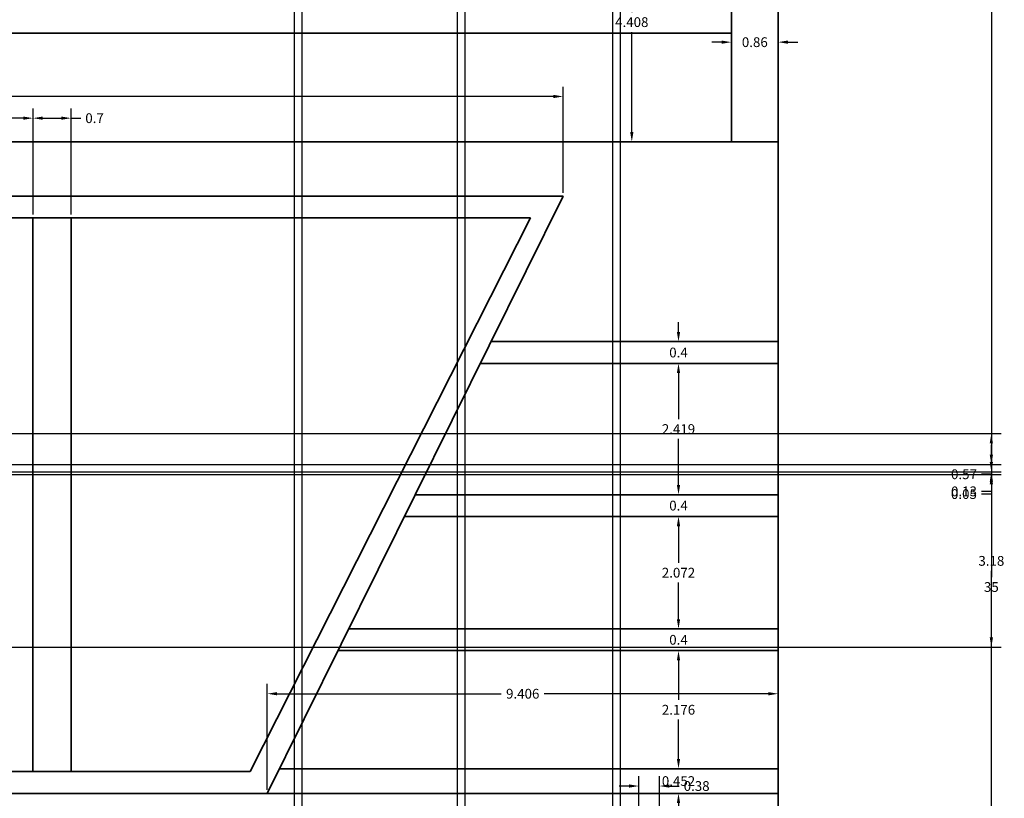
# Model space of a CAD drawing. Units: millimetres. Extents: x 2473 to 2512.3, y 2191.3 to 2230.4.
# Tile 7 of 8: x 2493.7 to 2511.8, y 2207 to 2221.3. Entities that reach past the tile are written whole.
import ezdxf

# ---------------------------------------------------------------- set-up
doc = ezdxf.new("R2010")
doc.units = ezdxf.units.MM
doc.layers.add('A-ANNO-DIMS', color=2, linetype='Continuous', lineweight=18)
doc.layers.add('A-ELEV', color=7, linetype='Continuous', lineweight=35)
doc.styles.get("Standard").update_dxf_attribs({"font": 'arial.ttf'})
doc.dimstyles.get("Standard").update_dxf_attribs({"dimtxt": 0.18, "dimasz": 0.18, "dimexe": 0.18, "dimexo": 0.0625, "dimgap": 0.09, "dimtad": 0, "dimtih": 1, "dimtoh": 1, "dimdec": 4, "dimzin": 0, "dimdsep": 46, "dimtxsty": 'Standard', "dimcen": 0.09, "dimadec": 0, "dimazin": 0, "dimtfac": 1, "dimtdec": 4, "dimtofl": 0, "dimtmove": 0, "dimatfit": 3, "dimfxl": 1, "dimtolj": 1, "dimtzin": 0, "dimarcsym": 0})

# ---------------------------------------------------------------- blocks, each defined once
blk = doc.blocks.new('*D9')
at = {"layer": 'A-ANNO-DIMS', "color": 0, "lineweight": -2, "transparency": 16777216}
for p, q in [((2509.775, 2228.355), (2511.728, 2228.355)), ((2511.548, 2228.175), (2511.548, 2211.037)), ((2511.548, 2193.535), (2511.548, 2210.673)), ((2507.685, 2193.355), (2511.728, 2193.355))]:
    blk.add_line(p, q, dxfattribs=at)
at = {"layer": 'A-ANNO-DIMS', "color": 0, "transparency": 16777216}
for points in [[(2511.518, 2228.175), (2511.578, 2228.175), (2511.548, 2228.355)], [(2511.518, 2193.535), (2511.578, 2193.535), (2511.548, 2193.355)]]:
    blk.add_solid(points, dxfattribs=at)
at = {"layer": 'Defpoints', "color": 0, "transparency": 16777216}
for p in [(2509.713, 2228.355), (2511.548, 2228.355), (2507.623, 2193.355)]:
    blk.add_point(p, dxfattribs=at)
at = {"layer": 'A-ANNO-DIMS', "color": 0, "transparency": 16777216, "insert": (2511.548, 2210.855), "char_height": 0.18, "attachment_point": 5}
blk.add_mtext('\\A1;35', dxfattribs=at)
blk = doc.blocks.new('*D18')
at = {"layer": 'A-ANNO-DIMS', "color": 0, "lineweight": -2, "transparency": 16777216}
for p, q in [((2476.623, 2218.117), (2476.623, 2220.07)), ((2503.664, 2218.117), (2503.664, 2220.07)), ((2476.803, 2219.89), (2489.749, 2219.89)), ((2503.484, 2219.89), (2490.538, 2219.89))]:
    blk.add_line(p, q, dxfattribs=at)
at = {"layer": 'A-ANNO-DIMS', "color": 0, "transparency": 16777216}
for points in [[(2476.803, 2219.92), (2476.803, 2219.86), (2476.623, 2219.89)], [(2503.484, 2219.92), (2503.484, 2219.86), (2503.664, 2219.89)]]:
    blk.add_solid(points, dxfattribs=at)
at = {"layer": 'Defpoints', "color": 0, "transparency": 16777216}
for p in [(2503.664, 2219.89), (2476.623, 2218.055), (2503.664, 2218.055)]:
    blk.add_point(p, dxfattribs=at)
at = {"layer": 'A-ANNO-DIMS', "color": 0, "transparency": 16777216, "insert": (2490.143, 2219.89), "char_height": 0.18, "attachment_point": 5}
blk.add_mtext('\\A1;27.04', dxfattribs=at)
blk = doc.blocks.new('*D31')
at = {"layer": 'A-ANNO-DIMS', "color": 0, "lineweight": -2, "transparency": 16777216}
for p, q in [((2505.056, 2205.417), (2505.056, 2207.37)), ((2505.438, 2205.417), (2505.438, 2207.37)), ((2504.876, 2207.19), (2504.696, 2207.19)), ((2505.618, 2207.19), (2505.798, 2207.19))]:
    blk.add_line(p, q, dxfattribs=at)
at = {"layer": 'A-ANNO-DIMS', "color": 0, "transparency": 16777216}
for points in [[(2504.876, 2207.22), (2504.876, 2207.16), (2505.056, 2207.19)], [(2505.618, 2207.22), (2505.618, 2207.16), (2505.438, 2207.19)]]:
    blk.add_solid(points, dxfattribs=at)
at = {"layer": 'Defpoints', "color": 0, "transparency": 16777216}
for p in [(2505.438, 2207.19), (2505.056, 2205.355), (2505.438, 2205.355)]:
    blk.add_point(p, dxfattribs=at)
at = {"layer": 'A-ANNO-DIMS', "color": 0, "transparency": 16777216, "insert": (2506.122, 2207.19), "char_height": 0.18, "attachment_point": 5}
blk.add_mtext('\\A1;0.38', dxfattribs=at)
blk = doc.blocks.new('*D46')
at = {"layer": 'A-ANNO-DIMS', "color": 0, "lineweight": -2, "transparency": 16777216}
for p, q in [((2498.217, 2207.117), (2498.217, 2209.07)), ((2498.397, 2208.89), (2502.526, 2208.89)), ((2507.443, 2208.89), (2503.313, 2208.89)), ((2507.623, 2207.117), (2507.623, 2209.07))]:
    blk.add_line(p, q, dxfattribs=at)
at = {"layer": 'A-ANNO-DIMS', "color": 0, "transparency": 16777216}
for points in [[(2498.397, 2208.92), (2498.397, 2208.86), (2498.217, 2208.89)], [(2507.443, 2208.92), (2507.443, 2208.86), (2507.623, 2208.89)]]:
    blk.add_solid(points, dxfattribs=at)
at = {"layer": 'Defpoints', "color": 0, "transparency": 16777216}
for p in [(2507.623, 2208.89), (2498.217, 2207.055), (2507.623, 2207.055)]:
    blk.add_point(p, dxfattribs=at)
at = {"layer": 'A-ANNO-DIMS', "color": 0, "transparency": 16777216, "insert": (2502.92, 2208.89), "char_height": 0.18, "attachment_point": 5}
blk.add_mtext('\\A1;9.406', dxfattribs=at)
blk = doc.blocks.new('*D50')
at = {"layer": 'A-ANNO-DIMS', "color": 0, "lineweight": -2, "transparency": 16777216}
for p, q in [((2491.904, 2217.717), (2491.904, 2219.67)), ((2493.904, 2217.717), (2493.904, 2219.67)), ((2492.084, 2219.49), (2492.754, 2219.49)), ((2493.724, 2219.49), (2493.053, 2219.49))]:
    blk.add_line(p, q, dxfattribs=at)
at = {"layer": 'A-ANNO-DIMS', "color": 0, "transparency": 16777216}
for points in [[(2492.084, 2219.52), (2492.084, 2219.46), (2491.904, 2219.49)], [(2493.724, 2219.52), (2493.724, 2219.46), (2493.904, 2219.49)]]:
    blk.add_solid(points, dxfattribs=at)
at = {"layer": 'Defpoints', "color": 0, "transparency": 16777216}
for p in [(2493.904, 2219.49), (2491.904, 2217.655), (2493.904, 2217.655)]:
    blk.add_point(p, dxfattribs=at)
at = {"layer": 'A-ANNO-DIMS', "color": 0, "transparency": 16777216, "insert": (2492.904, 2219.49), "char_height": 0.18, "attachment_point": 5}
blk.add_mtext('\\A1;2', dxfattribs=at)
blk = doc.blocks.new('*D51')
at = {"layer": 'A-ANNO-DIMS', "color": 0, "lineweight": -2, "transparency": 16777216}
for p, q in [((2493.904, 2217.717), (2493.904, 2219.67)), ((2494.604, 2217.717), (2494.604, 2219.67)), ((2494.084, 2219.49), (2494.424, 2219.49)), ((2494.604, 2219.49), (2494.784, 2219.49))]:
    blk.add_line(p, q, dxfattribs=at)
at = {"layer": 'A-ANNO-DIMS', "color": 0, "transparency": 16777216}
for points in [[(2494.084, 2219.52), (2494.084, 2219.46), (2493.904, 2219.49)], [(2494.424, 2219.52), (2494.424, 2219.46), (2494.604, 2219.49)]]:
    blk.add_solid(points, dxfattribs=at)
at = {"layer": 'Defpoints', "color": 0, "transparency": 16777216}
for p in [(2494.604, 2219.49), (2493.904, 2217.655), (2494.604, 2217.655)]:
    blk.add_point(p, dxfattribs=at)
at = {"layer": 'A-ANNO-DIMS', "color": 0, "transparency": 16777216, "insert": (2495.037, 2219.49), "char_height": 0.18, "attachment_point": 5}
blk.add_mtext('\\A1;0.7', dxfattribs=at)
blk = doc.blocks.new('*D61')
at = {"layer": 'A-ANNO-DIMS', "color": 0, "lineweight": -2, "transparency": 16777216}
for p, q in [((2505.788, 2207.687), (2505.788, 2207.867)), ((2507.56, 2207.507), (2505.608, 2207.507)), ((2507.56, 2207.055), (2505.608, 2207.055)), ((2505.788, 2206.875), (2505.788, 2206.695))]:
    blk.add_line(p, q, dxfattribs=at)
at = {"layer": 'A-ANNO-DIMS', "color": 0, "transparency": 16777216}
for points in [[(2505.758, 2207.687), (2505.818, 2207.687), (2505.788, 2207.507)], [(2505.758, 2206.875), (2505.818, 2206.875), (2505.788, 2207.055)]]:
    blk.add_solid(points, dxfattribs=at)
at = {"layer": 'Defpoints', "color": 0, "transparency": 16777216}
for p in [(2505.788, 2207.507), (2507.623, 2207.507), (2507.623, 2207.055)]:
    blk.add_point(p, dxfattribs=at)
at = {"layer": 'A-ANNO-DIMS', "color": 0, "transparency": 16777216, "insert": (2505.788, 2207.281), "char_height": 0.18, "attachment_point": 5}
blk.add_mtext('\\A1;0.452', dxfattribs=at)
blk = doc.blocks.new('*D62')
at = {"layer": 'A-ANNO-DIMS', "color": 0, "lineweight": -2, "transparency": 16777216}
for p, q in [((2507.56, 2209.683), (2505.608, 2209.683)), ((2505.788, 2209.503), (2505.788, 2208.777)), ((2505.788, 2207.687), (2505.788, 2208.413)), ((2507.56, 2207.507), (2505.608, 2207.507))]:
    blk.add_line(p, q, dxfattribs=at)
at = {"layer": 'A-ANNO-DIMS', "color": 0, "transparency": 16777216}
for points in [[(2505.758, 2209.503), (2505.818, 2209.503), (2505.788, 2209.683)], [(2505.758, 2207.687), (2505.818, 2207.687), (2505.788, 2207.507)]]:
    blk.add_solid(points, dxfattribs=at)
at = {"layer": 'Defpoints', "color": 0, "transparency": 16777216}
for p in [(2505.788, 2209.683), (2507.623, 2209.683), (2507.623, 2207.507)]:
    blk.add_point(p, dxfattribs=at)
at = {"layer": 'A-ANNO-DIMS', "color": 0, "transparency": 16777216, "insert": (2505.788, 2208.595), "char_height": 0.18, "attachment_point": 5}
blk.add_mtext('\\A1;2.176', dxfattribs=at)
blk = doc.blocks.new('*D63')
at = {"layer": 'A-ANNO-DIMS', "color": 0, "lineweight": -2, "transparency": 16777216}
for p, q in [((2505.787904, 2210.263087), (2505.787904, 2210.443087)), ((2507.560404, 2210.083087), (2505.607904, 2210.083087)), ((2507.560404, 2209.683087), (2505.607904, 2209.683087)), ((2505.787904, 2209.503087), (2505.787904, 2209.323087))]:
    blk.add_line(p, q, dxfattribs=at)
at = {"layer": 'A-ANNO-DIMS', "color": 0, "transparency": 16777216}
for points in [[(2505.757904, 2210.263087), (2505.817904, 2210.263087), (2505.787904, 2210.083087)], [(2505.757904, 2209.503087), (2505.817904, 2209.503087), (2505.787904, 2209.683087)]]:
    blk.add_solid(points, dxfattribs=at)
at = {"layer": 'Defpoints', "color": 0, "transparency": 16777216}
for p in [(2505.787904, 2210.083087), (2507.622904, 2210.083087), (2507.622904, 2209.683087)]:
    blk.add_point(p, dxfattribs=at)
at = {"layer": 'A-ANNO-DIMS', "color": 0, "transparency": 16777216, "insert": (2505.787904, 2209.883087), "char_height": 0.18, "attachment_point": 5}
blk.add_mtext('\\A1;0.4', dxfattribs=at)
blk = doc.blocks.new('*D64')
at = {"layer": 'A-ANNO-DIMS', "color": 0, "lineweight": -2, "transparency": 16777216}
for p, q in [((2507.56, 2212.155), (2505.608, 2212.155)), ((2505.788, 2211.975), (2505.788, 2211.301)), ((2505.788, 2210.263), (2505.788, 2210.937)), ((2507.56, 2210.083), (2505.608, 2210.083))]:
    blk.add_line(p, q, dxfattribs=at)
at = {"layer": 'A-ANNO-DIMS', "color": 0, "transparency": 16777216}
for points in [[(2505.758, 2211.975), (2505.818, 2211.975), (2505.788, 2212.155)], [(2505.758, 2210.263), (2505.818, 2210.263), (2505.788, 2210.083)]]:
    blk.add_solid(points, dxfattribs=at)
at = {"layer": 'Defpoints', "color": 0, "transparency": 16777216}
for p in [(2505.788, 2212.155), (2507.623, 2212.155), (2507.623, 2210.083)]:
    blk.add_point(p, dxfattribs=at)
at = {"layer": 'A-ANNO-DIMS', "color": 0, "transparency": 16777216, "insert": (2505.788, 2211.119), "char_height": 0.18, "attachment_point": 5}
blk.add_mtext('\\A1;2.072', dxfattribs=at)
blk = doc.blocks.new('*D65')
at = {"layer": 'A-ANNO-DIMS', "color": 0, "lineweight": -2, "transparency": 16777216}
for p, q in [((2505.787904, 2212.734888), (2505.787904, 2212.914888)), ((2507.560404, 2212.554888), (2505.607904, 2212.554888)), ((2507.560404, 2212.154888), (2505.607904, 2212.154888)), ((2505.787904, 2211.974888), (2505.787904, 2211.794888))]:
    blk.add_line(p, q, dxfattribs=at)
at = {"layer": 'A-ANNO-DIMS', "color": 0, "transparency": 16777216}
for points in [[(2505.757904, 2212.734888), (2505.817904, 2212.734888), (2505.787904, 2212.554888)], [(2505.757904, 2211.974888), (2505.817904, 2211.974888), (2505.787904, 2212.154888)]]:
    blk.add_solid(points, dxfattribs=at)
at = {"layer": 'Defpoints', "color": 0, "transparency": 16777216}
for p in [(2505.787904, 2212.554888), (2507.622904, 2212.554888), (2507.622904, 2212.154888)]:
    blk.add_point(p, dxfattribs=at)
at = {"layer": 'A-ANNO-DIMS', "color": 0, "transparency": 16777216, "insert": (2505.787904, 2212.354888), "char_height": 0.18, "attachment_point": 5}
blk.add_mtext('\\A1;0.4', dxfattribs=at)
blk = doc.blocks.new('*D66')
at = {"layer": 'A-ANNO-DIMS', "color": 0, "lineweight": -2, "transparency": 16777216}
for p, q in [((2507.56, 2214.974), (2505.608, 2214.974)), ((2505.788, 2214.794), (2505.788, 2213.946)), ((2505.788, 2212.735), (2505.788, 2213.583)), ((2507.56, 2212.555), (2505.608, 2212.555))]:
    blk.add_line(p, q, dxfattribs=at)
at = {"layer": 'A-ANNO-DIMS', "color": 0, "transparency": 16777216}
for points in [[(2505.758, 2214.794), (2505.818, 2214.794), (2505.788, 2214.974)], [(2505.758, 2212.735), (2505.818, 2212.735), (2505.788, 2212.555)]]:
    blk.add_solid(points, dxfattribs=at)
at = {"layer": 'Defpoints', "color": 0, "transparency": 16777216}
for p in [(2505.788, 2214.974), (2507.623, 2214.974), (2507.623, 2212.555)]:
    blk.add_point(p, dxfattribs=at)
at = {"layer": 'A-ANNO-DIMS', "color": 0, "transparency": 16777216, "insert": (2505.788, 2213.764), "char_height": 0.18, "attachment_point": 5}
blk.add_mtext('\\A1;2.419', dxfattribs=at)
blk = doc.blocks.new('*D67')
at = {"layer": 'A-ANNO-DIMS', "color": 0, "lineweight": -2, "transparency": 16777216}
for p, q in [((2505.787904, 2215.553995), (2505.787904, 2215.733995)), ((2507.560404, 2215.373995), (2505.607904, 2215.373995)), ((2507.560404, 2214.973995), (2505.607904, 2214.973995)), ((2505.787904, 2214.793995), (2505.787904, 2214.613995))]:
    blk.add_line(p, q, dxfattribs=at)
at = {"layer": 'A-ANNO-DIMS', "color": 0, "transparency": 16777216}
for points in [[(2505.757904, 2215.553995), (2505.817904, 2215.553995), (2505.787904, 2215.373995)], [(2505.757904, 2214.793995), (2505.817904, 2214.793995), (2505.787904, 2214.973995)]]:
    blk.add_solid(points, dxfattribs=at)
at = {"layer": 'Defpoints', "color": 0, "transparency": 16777216}
for p in [(2505.787904, 2215.373995), (2507.622904, 2215.373995), (2507.622904, 2214.973995)]:
    blk.add_point(p, dxfattribs=at)
at = {"layer": 'A-ANNO-DIMS', "color": 0, "transparency": 16777216, "insert": (2505.787904, 2215.173995), "char_height": 0.18, "attachment_point": 5}
blk.add_mtext('\\A1;0.4', dxfattribs=at)
blk = doc.blocks.new('*D89')
at = {"layer": 'A-ANNO-DIMS', "color": 0, "lineweight": -2, "transparency": 16777216}
for p, q in [((2506.763, 2219.117), (2506.763, 2221.07)), ((2507.623, 2219.117), (2507.623, 2221.07)), ((2506.583, 2220.89), (2506.403, 2220.89)), ((2507.803, 2220.89), (2507.983, 2220.89))]:
    blk.add_line(p, q, dxfattribs=at)
at = {"layer": 'A-ANNO-DIMS', "color": 0, "transparency": 16777216}
for points in [[(2506.583, 2220.92), (2506.583, 2220.86), (2506.763, 2220.89)], [(2507.803, 2220.92), (2507.803, 2220.86), (2507.623, 2220.89)]]:
    blk.add_solid(points, dxfattribs=at)
at = {"layer": 'Defpoints', "color": 0, "transparency": 16777216}
for p in [(2507.623, 2220.89), (2506.763, 2219.055), (2507.623, 2219.055)]:
    blk.add_point(p, dxfattribs=at)
at = {"layer": 'A-ANNO-DIMS', "color": 0, "transparency": 16777216, "insert": (2507.193, 2220.89), "char_height": 0.18, "attachment_point": 5}
blk.add_mtext('\\A1;0.86', dxfattribs=at)
blk = doc.blocks.new('*D91')
at = {"layer": 'A-ANNO-DIMS', "color": 0, "lineweight": -2, "transparency": 16777216}
for p, q in [((2506.7, 2223.463), (2504.748, 2223.463)), ((2504.928, 2223.283), (2504.928, 2221.441)), ((2504.928, 2219.235), (2504.928, 2221.077)), ((2506.7, 2219.055), (2504.748, 2219.055))]:
    blk.add_line(p, q, dxfattribs=at)
at = {"layer": 'A-ANNO-DIMS', "color": 0, "transparency": 16777216}
for points in [[(2504.898, 2223.283), (2504.958, 2223.283), (2504.928, 2223.463)], [(2504.898, 2219.235), (2504.958, 2219.235), (2504.928, 2219.055)]]:
    blk.add_solid(points, dxfattribs=at)
at = {"layer": 'Defpoints', "color": 0, "transparency": 16777216}
for p in [(2504.928, 2223.463), (2506.763, 2223.463), (2506.763, 2219.055)]:
    blk.add_point(p, dxfattribs=at)
at = {"layer": 'A-ANNO-DIMS', "color": 0, "transparency": 16777216, "insert": (2504.928, 2221.259), "char_height": 0.18, "attachment_point": 5}
blk.add_mtext('\\A1;4.408', dxfattribs=at)
blk = doc.blocks.new('*D111')
at = {"layer": 'A-ANNO-DIMS', "color": 0, "lineweight": -2, "transparency": 16777216}
for p, q in [((2486.902, 2213.68), (2511.728, 2213.68)), ((2511.548, 2213.5), (2511.548, 2213.292)), ((2486.718, 2213.112), (2511.728, 2213.112)), ((2511.548, 2213.112), (2511.548, 2212.932)), ((2511.548, 2212.932), (2511.368, 2212.932))]:
    blk.add_line(p, q, dxfattribs=at)
at = {"layer": 'A-ANNO-DIMS', "color": 0, "transparency": 16777216}
for points in [[(2511.518, 2213.5), (2511.578, 2213.5), (2511.548, 2213.68)], [(2511.518, 2213.292), (2511.578, 2213.292), (2511.548, 2213.112)]]:
    blk.add_solid(points, dxfattribs=at)
at = {"layer": 'Defpoints', "color": 0, "transparency": 16777216}
for p in [(2486.84, 2213.68), (2486.655, 2213.112), (2511.548, 2213.112)]:
    blk.add_point(p, dxfattribs=at)
at = {"layer": 'A-ANNO-DIMS', "color": 0, "transparency": 16777216, "insert": (2511.044, 2212.932), "char_height": 0.18, "attachment_point": 5}
blk.add_mtext('\\A1;0.57', dxfattribs=at)
blk = doc.blocks.new('*D112')
at = {"layer": 'A-ANNO-DIMS', "color": 0, "lineweight": -2, "transparency": 16777216}
for p, q in [((2511.548, 2213.292), (2511.548, 2213.472)), ((2486.718, 2213.112), (2511.728, 2213.112)), ((2486.625, 2212.977), (2511.728, 2212.977)), ((2511.548, 2212.797), (2511.548, 2212.617)), ((2511.548, 2212.617), (2511.368, 2212.617))]:
    blk.add_line(p, q, dxfattribs=at)
at = {"layer": 'A-ANNO-DIMS', "color": 0, "transparency": 16777216}
for points in [[(2511.518, 2213.292), (2511.578, 2213.292), (2511.548, 2213.112)], [(2511.518, 2212.797), (2511.578, 2212.797), (2511.548, 2212.977)]]:
    blk.add_solid(points, dxfattribs=at)
at = {"layer": 'Defpoints', "color": 0, "transparency": 16777216}
for p in [(2486.655, 2213.112), (2486.562, 2212.977), (2511.548, 2212.977)]:
    blk.add_point(p, dxfattribs=at)
at = {"layer": 'A-ANNO-DIMS', "color": 0, "transparency": 16777216, "insert": (2511.044, 2212.617), "char_height": 0.18, "attachment_point": 5}
blk.add_mtext('\\A1;0.13', dxfattribs=at)
blk = doc.blocks.new('*D113')
at = {"layer": 'A-ANNO-DIMS', "color": 0, "lineweight": -2, "transparency": 16777216}
for p, q in [((2511.548, 2213.157), (2511.548, 2213.337)), ((2486.583, 2212.927), (2511.728, 2212.927)), ((2486.625, 2212.977), (2511.728, 2212.977)), ((2511.548, 2212.747), (2511.548, 2212.567)), ((2511.548, 2212.567), (2511.368, 2212.567))]:
    blk.add_line(p, q, dxfattribs=at)
at = {"layer": 'A-ANNO-DIMS', "color": 0, "transparency": 16777216}
for points in [[(2511.518, 2213.157), (2511.578, 2213.157), (2511.548, 2212.977)], [(2511.518, 2212.747), (2511.578, 2212.747), (2511.548, 2212.927)]]:
    blk.add_solid(points, dxfattribs=at)
at = {"layer": 'Defpoints', "color": 0, "transparency": 16777216}
for p in [(2486.52, 2212.927), (2486.562, 2212.977), (2511.548, 2212.927)]:
    blk.add_point(p, dxfattribs=at)
at = {"layer": 'A-ANNO-DIMS', "color": 0, "transparency": 16777216, "insert": (2511.043, 2212.567), "char_height": 0.18, "attachment_point": 5}
blk.add_mtext('\\A1;0.05', dxfattribs=at)
blk = doc.blocks.new('*D114')
at = {"layer": 'A-ANNO-DIMS', "color": 0, "lineweight": -2, "transparency": 16777216}
for p, q in [((2486.583, 2212.927), (2511.728, 2212.927)), ((2511.548, 2212.747), (2511.548, 2211.519)), ((2511.548, 2209.927), (2511.548, 2211.155)), ((2486.583, 2209.747), (2511.728, 2209.747))]:
    blk.add_line(p, q, dxfattribs=at)
at = {"layer": 'A-ANNO-DIMS', "color": 0, "transparency": 16777216}
for points in [[(2511.518, 2212.747), (2511.578, 2212.747), (2511.548, 2212.927)], [(2511.518, 2209.927), (2511.578, 2209.927), (2511.548, 2209.747)]]:
    blk.add_solid(points, dxfattribs=at)
at = {"layer": 'Defpoints', "color": 0, "transparency": 16777216}
for p in [(2486.52, 2212.927), (2486.52, 2209.747), (2511.548, 2209.747)]:
    blk.add_point(p, dxfattribs=at)
at = {"layer": 'A-ANNO-DIMS', "color": 0, "transparency": 16777216, "insert": (2511.548, 2211.337), "char_height": 0.18, "attachment_point": 5}
blk.add_mtext('\\A1;3.18', dxfattribs=at)
blk = doc.blocks.new('*D115')
at = {"layer": 'A-ANNO-DIMS', "color": 0, "lineweight": -2, "transparency": 16777216}
for p, q in [((2498.713, 2222.992), (2498.713, 2191.34)), ((2498.852, 2222.992), (2498.852, 2191.34)), ((2498.533, 2191.52), (2498.353, 2191.52)), ((2499.032, 2191.52), (2499.212, 2191.52))]:
    blk.add_line(p, q, dxfattribs=at)
at = {"layer": 'A-ANNO-DIMS', "color": 0, "transparency": 16777216}
for points in [[(2498.533, 2191.55), (2498.533, 2191.49), (2498.713, 2191.52)], [(2499.032, 2191.55), (2499.032, 2191.49), (2498.852, 2191.52)]]:
    blk.add_solid(points, dxfattribs=at)
at = {"layer": 'Defpoints', "color": 0, "transparency": 16777216}
for p in [(2498.713, 2223.055), (2498.852, 2223.055), (2498.852, 2191.52)]:
    blk.add_point(p, dxfattribs=at)
at = {"layer": 'A-ANNO-DIMS', "color": 0, "transparency": 16777216, "insert": (2499.536, 2191.52), "char_height": 0.18, "attachment_point": 5}
blk.add_mtext('\\A1;0.14', dxfattribs=at)
blk = doc.blocks.new('*D116')
at = {"layer": 'A-ANNO-DIMS', "color": 0, "lineweight": -2, "transparency": 16777216}
for p, q in [((2498.852, 2222.992), (2498.852, 2191.34)), ((2501.713, 2222.992), (2501.713, 2191.34)), ((2499.032, 2191.52), (2499.957, 2191.52)), ((2501.533, 2191.52), (2500.608, 2191.52))]:
    blk.add_line(p, q, dxfattribs=at)
at = {"layer": 'A-ANNO-DIMS', "color": 0, "transparency": 16777216}
for points in [[(2499.032, 2191.55), (2499.032, 2191.49), (2498.852, 2191.52)], [(2501.533, 2191.55), (2501.533, 2191.49), (2501.713, 2191.52)]]:
    blk.add_solid(points, dxfattribs=at)
at = {"layer": 'Defpoints', "color": 0, "transparency": 16777216}
for p in [(2498.852, 2223.055), (2501.713, 2223.055), (2501.713, 2191.52)]:
    blk.add_point(p, dxfattribs=at)
at = {"layer": 'A-ANNO-DIMS', "color": 0, "transparency": 16777216, "insert": (2500.283, 2191.52), "char_height": 0.18, "attachment_point": 5}
blk.add_mtext('\\A1;2.86', dxfattribs=at)
blk = doc.blocks.new('*D117')
at = {"layer": 'A-ANNO-DIMS', "color": 0, "lineweight": -2, "transparency": 16777216}
for p, q in [((2501.713, 2222.992), (2501.713, 2191.34)), ((2501.853, 2222.992), (2501.853, 2191.34)), ((2501.533, 2191.52), (2501.353, 2191.52)), ((2502.033, 2191.52), (2502.213, 2191.52))]:
    blk.add_line(p, q, dxfattribs=at)
at = {"layer": 'A-ANNO-DIMS', "color": 0, "transparency": 16777216}
for points in [[(2501.533, 2191.55), (2501.533, 2191.49), (2501.713, 2191.52)], [(2502.033, 2191.55), (2502.033, 2191.49), (2501.853, 2191.52)]]:
    blk.add_solid(points, dxfattribs=at)
at = {"layer": 'Defpoints', "color": 0, "transparency": 16777216}
for p in [(2501.713, 2223.055), (2501.853, 2223.055), (2501.853, 2191.52)]:
    blk.add_point(p, dxfattribs=at)
at = {"layer": 'A-ANNO-DIMS', "color": 0, "transparency": 16777216, "insert": (2502.536, 2191.52), "char_height": 0.18, "attachment_point": 5}
blk.add_mtext('\\A1;0.14', dxfattribs=at)
blk = doc.blocks.new('*D118')
at = {"layer": 'A-ANNO-DIMS', "color": 0, "lineweight": -2, "transparency": 16777216}
for p, q in [((2501.853, 2222.992), (2501.853, 2191.34)), ((2504.573, 2222.992), (2504.573, 2191.34)), ((2502.033, 2191.52), (2502.888, 2191.52)), ((2504.393, 2191.52), (2503.537, 2191.52))]:
    blk.add_line(p, q, dxfattribs=at)
at = {"layer": 'A-ANNO-DIMS', "color": 0, "transparency": 16777216}
for points in [[(2502.033, 2191.55), (2502.033, 2191.49), (2501.853, 2191.52)], [(2504.393, 2191.55), (2504.393, 2191.49), (2504.573, 2191.52)]]:
    blk.add_solid(points, dxfattribs=at)
at = {"layer": 'Defpoints', "color": 0, "transparency": 16777216}
for p in [(2501.853, 2223.055), (2504.573, 2223.055), (2504.573, 2191.52)]:
    blk.add_point(p, dxfattribs=at)
at = {"layer": 'A-ANNO-DIMS', "color": 0, "transparency": 16777216, "insert": (2503.213, 2191.52), "char_height": 0.18, "attachment_point": 5}
blk.add_mtext('\\A1;2.72', dxfattribs=at)
blk = doc.blocks.new('*D119')
at = {"layer": 'A-ANNO-DIMS', "color": 0, "lineweight": -2, "transparency": 16777216}
for p, q in [((2504.573, 2222.992), (2504.573, 2191.34)), ((2504.713, 2222.992), (2504.713, 2191.34)), ((2504.393, 2191.52), (2504.213, 2191.52)), ((2504.893, 2191.52), (2505.073, 2191.52))]:
    blk.add_line(p, q, dxfattribs=at)
at = {"layer": 'A-ANNO-DIMS', "color": 0, "transparency": 16777216}
for points in [[(2504.393, 2191.55), (2504.393, 2191.49), (2504.573, 2191.52)], [(2504.893, 2191.55), (2504.893, 2191.49), (2504.713, 2191.52)]]:
    blk.add_solid(points, dxfattribs=at)
at = {"layer": 'Defpoints', "color": 0, "transparency": 16777216}
for p in [(2504.573, 2223.055), (2504.713, 2223.055), (2504.713, 2191.52)]:
    blk.add_point(p, dxfattribs=at)
at = {"layer": 'A-ANNO-DIMS', "color": 0, "transparency": 16777216, "insert": (2505.396, 2191.52), "char_height": 0.18, "attachment_point": 5}
blk.add_mtext('\\A1;0.14', dxfattribs=at)

msp = doc.modelspace()

# ---------------------------------------------------------------- linework, layer by layer
at = {"layer": 'A-ELEV'}
for p, q in [((2506.7629, 2219.0549), (2506.7629, 2223.4627)), ((2507.6229, 2223.0549), (2507.6229, 2219.0549)), ((2506.7629, 2221.0549), (2475.6229, 2221.0549)), ((2506.7629, 2219.0549), (2475.6229, 2219.0549)), ((2507.6229, 2219.0549), (2506.7629, 2219.0549)), ((2507.6229, 2219.0549), (2507.6229, 2193.3549)), ((2503.6639, 2218.0549), (2476.6229, 2218.0549)), ((2498.2167, 2207.0549), (2503.6639, 2218.0549)), ((2477.0229, 2217.6549), (2503.0616, 2217.6549)), ((2493.9035, 2207.4549), (2493.9035, 2217.6549)), ((2494.6035, 2217.6549), (2494.6035, 2207.4549)), ((2503.0616, 2217.6549), (2497.9035, 2207.4549)), ((2502.3363, 2215.374), (2507.6229, 2215.374)), ((2502.3363, 2214.974), (2502.1383, 2214.974)), ((2502.3363, 2214.974), (2507.6229, 2214.974)), ((2500.9403, 2212.5549), (2507.6229, 2212.5549)), ((2500.9403, 2212.1549), (2500.7422, 2212.1549)), ((2500.9403, 2212.1549), (2507.6229, 2212.1549)), ((2499.7163, 2210.0831), (2507.6229, 2210.0831)), ((2499.7163, 2209.6831), (2499.5182, 2209.6831)), ((2499.7163, 2209.6831), (2507.6229, 2209.6831)), ((2477.0229, 2207.4549), (2497.9035, 2207.4549)), ((2498.4405, 2207.5069), (2507.6229, 2207.5069)), ((2476.6229, 2207.0549), (2498.2167, 2207.0549)), ((2498.2167, 2207.0549), (2507.6229, 2207.0549))]:
    msp.add_line(p, q, dxfattribs=at)

# ---------------------------------------------------------------- dimensions: what is measured, and where the dimension line sits
at = {"layer": 'A-ANNO-DIMS'}
for base, p1, p2, override, picture, middle in [((2511.5479, 2228.3549), (2507.6229, 2193.3549), (2509.7129, 2228.3549), {"dimdec": 0, "dimlfac": 1, "dimrnd": 0, "dimzin": 0, "dimdsep": 46, "dimlunit": 2}, '*D9', (2511.5479, 2210.8549)), ((2504.9279, 2223.4627), (2506.7629, 2219.0549), (2506.7629, 2223.4627), {"dimdec": 3, "dimlfac": 1, "dimrnd": 0, "dimzin": 0, "dimdsep": 46, "dimlunit": 2}, '*D91', (2504.9279, 2221.2588)), ((2505.7879, 2215.374), (2507.6229, 2214.974), (2507.6229, 2215.374), {"dimdec": 1, "dimlfac": 1, "dimrnd": 0, "dimzin": 0, "dimdsep": 46, "dimlunit": 2}, '*D67', (2505.7879, 2215.174)), ((2505.7879, 2214.974), (2507.6229, 2212.5549), (2507.6229, 2214.974), {"dimdec": 3, "dimlfac": 1, "dimrnd": 0, "dimzin": 0, "dimdsep": 46, "dimlunit": 2}, '*D66', (2505.7879, 2213.7644)), ((2511.5479, 2213.1115), (2486.8395, 2213.6797), (2486.655, 2213.1115), {"dimdec": 2, "dimlfac": 1, "dimrnd": 0, "dimzin": 0, "dimdsep": 46, "dimlunit": 2}, '*D111', (2511.0441, 2212.9315)), ((2511.5479, 2212.9771), (2486.655, 2213.1115), (2486.5624, 2212.9771), {"dimdec": 2, "dimlfac": 1, "dimrnd": 0, "dimzin": 0, "dimdsep": 46, "dimlunit": 2}, '*D112', (2511.0441, 2212.6171)), ((2511.5479, 2212.9269), (2486.5624, 2212.9771), (2486.5205, 2212.9269), {"dimdec": 2, "dimlfac": 1, "dimrnd": 0, "dimzin": 0, "dimdsep": 46, "dimlunit": 2}, '*D113', (2511.0434, 2212.5669)), ((2511.5479, 2209.7466), (2486.5205, 2212.9269), (2486.5205, 2209.7466), {"dimdec": 2, "dimlfac": 1, "dimrnd": 0, "dimzin": 0, "dimdsep": 46, "dimlunit": 2}, '*D114', (2511.5479, 2211.3367)), ((2505.7879, 2212.5549), (2507.6229, 2212.1549), (2507.6229, 2212.5549), {"dimdec": 1, "dimlfac": 1, "dimrnd": 0, "dimzin": 0, "dimdsep": 46, "dimlunit": 2}, '*D65', (2505.7879, 2212.3549)), ((2505.7879, 2212.1549), (2507.6229, 2210.0831), (2507.6229, 2212.1549), {"dimdec": 3, "dimlfac": 1, "dimrnd": 0, "dimzin": 0, "dimdsep": 46, "dimlunit": 2}, '*D64', (2505.7879, 2211.119)), ((2505.7879, 2210.0831), (2507.6229, 2209.6831), (2507.6229, 2210.0831), {"dimdec": 1, "dimlfac": 1, "dimrnd": 0, "dimzin": 0, "dimdsep": 46, "dimlunit": 2}, '*D63', (2505.7879, 2209.8831)), ((2505.7879, 2209.6831), (2507.6229, 2207.5069), (2507.6229, 2209.6831), {"dimdec": 3, "dimlfac": 1, "dimrnd": 0, "dimzin": 0, "dimdsep": 46, "dimlunit": 2}, '*D62', (2505.7879, 2208.595)), ((2505.7879, 2207.5069), (2507.6229, 2207.0549), (2507.6229, 2207.5069), {"dimdec": 3, "dimlfac": 1, "dimrnd": 0, "dimzin": 0, "dimdsep": 46, "dimlunit": 2}, '*D61', (2505.7879, 2207.2809))]:
    dim = msp.add_linear_dim(base=base, p1=p1, p2=p2, angle=90, dimstyle='Standard', override=override, dxfattribs=at)
    dim.commit()
    dim.dimension.update_dxf_attribs({"geometry": picture, "text_midpoint": middle})
for base, p1, p2, override, picture, middle in [((2498.8524, 2191.5199), (2498.7129, 2223.0549), (2498.8524, 2223.0549), {"dimdec": 2, "dimlfac": 1, "dimrnd": 0, "dimzin": 0, "dimdsep": 46, "dimlunit": 2}, '*D115', (2499.5358, 2191.5199)), ((2501.7127, 2191.5199), (2498.8524, 2223.0549), (2501.7127, 2223.0549), {"dimdec": 2, "dimlfac": 1, "dimrnd": 0, "dimzin": 0, "dimdsep": 46, "dimlunit": 2}, '*D116', (2500.2825, 2191.5199)), ((2501.8527, 2191.5199), (2501.7127, 2223.0549), (2501.8527, 2223.0549), {"dimdec": 2, "dimlfac": 1, "dimrnd": 0, "dimzin": 0, "dimdsep": 46, "dimlunit": 2}, '*D117', (2502.5361, 2191.5199)), ((2504.5729, 2191.5199), (2501.8527, 2223.0549), (2504.5729, 2223.0549), {"dimdec": 2, "dimlfac": 1, "dimrnd": 0, "dimzin": 0, "dimdsep": 46, "dimlunit": 2}, '*D118', (2503.2128, 2191.5199)), ((2504.7129, 2191.5199), (2504.5729, 2223.0549), (2504.7129, 2223.0549), {"dimdec": 2, "dimlfac": 1, "dimrnd": 0, "dimzin": 0, "dimdsep": 46, "dimlunit": 2}, '*D119', (2505.3963, 2191.5199)), ((2507.6229, 2220.8899), (2506.7629, 2219.0549), (2507.6229, 2219.0549), {"dimdec": 2, "dimlfac": 1, "dimrnd": 0, "dimzin": 0, "dimdsep": 46, "dimlunit": 2}, '*D89', (2507.1929, 2220.8899)), ((2503.6639, 2219.8899), (2476.6229, 2218.0549), (2503.6639, 2218.0549), {"dimdec": 2, "dimlfac": 1, "dimrnd": 0, "dimzin": 0, "dimdsep": 46, "dimlunit": 2}, '*D18', (2490.1434, 2219.8899)), ((2493.9035, 2219.4899), (2491.9035, 2217.6549), (2493.9035, 2217.6549), {"dimdec": 0, "dimlfac": 1, "dimrnd": 0, "dimzin": 0, "dimdsep": 46, "dimlunit": 2}, '*D50', (2492.9035, 2219.4899)), ((2494.6035, 2219.4899), (2493.9035, 2217.6549), (2494.6035, 2217.6549), {"dimdec": 1, "dimlfac": 1, "dimrnd": 0, "dimzin": 0, "dimdsep": 46, "dimlunit": 2}, '*D51', (2495.0374, 2219.4899)), ((2507.6229, 2208.8899), (2498.2167, 2207.0549), (2507.6229, 2207.0549), {"dimdec": 3, "dimlfac": 1, "dimrnd": 0, "dimzin": 0, "dimdsep": 46, "dimlunit": 2}, '*D46', (2502.9198, 2208.8899)), ((2505.4377, 2207.1899), (2505.0565, 2205.3549), (2505.4377, 2205.3549), {"dimdec": 2, "dimlfac": 1, "dimrnd": 0, "dimzin": 0, "dimdsep": 46, "dimlunit": 2}, '*D31', (2506.1216, 2207.1899))]:
    dim = msp.add_linear_dim(base=base, p1=p1, p2=p2, dimstyle='Standard', override=override, dxfattribs=at)
    dim.commit()
    dim.dimension.update_dxf_attribs({"geometry": picture, "text_midpoint": middle})

doc.saveas('drawing.dxf')
